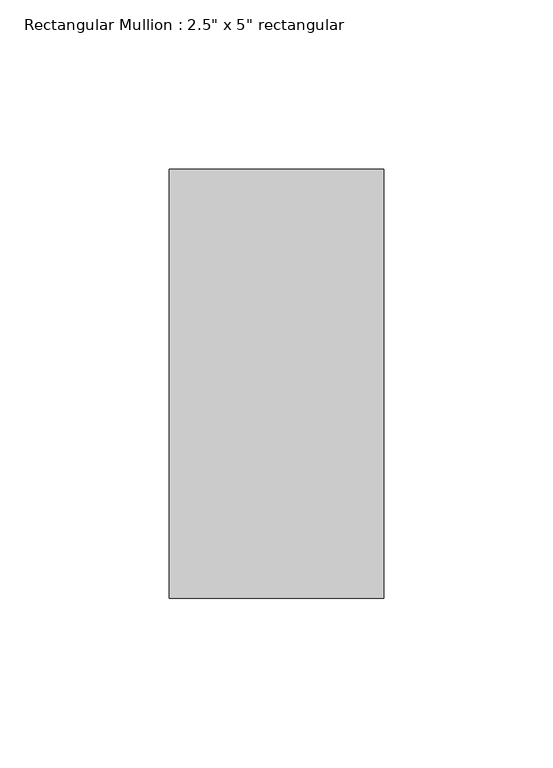
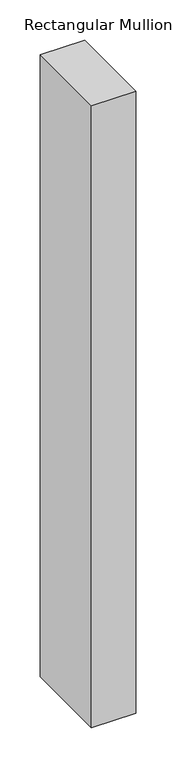
"""IFC4 building model written with IfcOpenShell, lengths in millimetres: member geometry."""

from ifc_helpers import new_model, si_unit, frame, origin, place, context, project, spatial, polyline, outline, extrude, source, transform, mapped, element, save


def member_e0b7b075(model_context):
    return source(origin(), model_context, "Body", "SweptSolid", [
        extrude(outline(polyline([(0.0, 63.5), (0.0, -63.5), (-63.5, -63.5), (-63.5, 63.5), (0.0, 63.5)])), frame((0.0, 0.0, -942.7710507), z_axis=(0.0, 0.0, 1.0), x_axis=(1.0, 0.0, 0.0)), (0.0, 0.0, 1.0), 942.7710507),
    ])


if __name__ == "__main__":
    model = new_model("IFC4")
    model_context = context("Model", 3, world=origin())
    ifc_project = project(units=[si_unit("LENGTHUNIT", "METRE", prefix="MILLI")], contexts=[model_context])
    site = spatial("IfcSite", under=ifc_project)
    building = spatial("IfcBuilding", under=site)
    placement = place(None, origin())
    member_shape = member_e0b7b075(model_context)
    element("IfcMember", 1, ObjectType="Rectangular Mullion : 2.5\" x 5\" rectangular", at=placement, inside=building, context=model_context, shape_type="MappedRepresentation", body=[
        mapped(member_shape, transform((0.0, 0.0, 0.0), x_axis=(1.0, 0.0, 0.0), y_axis=(0.0, 1.0, 0.0), z_axis=(0.0, 0.0, 1.0))),
    ])
    save(model, "model.ifc")

# Revit data of these elements
# Type "Rectangular Mullion : 2.5\" x 5\" rectangular"
#   built-in parameter 1007304 = 0.416667 (stored number, unit not read)
#   built-in parameter 1007301 = 0.104167 (stored number, unit not read)
#   built-in parameter 1007300 = 0.104167 (stored number, unit not read)
# Element 1 (IfcMember, "Rectangular Mullion : 2.5\" x 5\" rectangular")
#   Materials on its faces: "BLACK COLOUR"
# Materials
#   "BLACK COLOUR": class "Generic", colour RGB 120 120 120, transparency 0, Cost = 0
